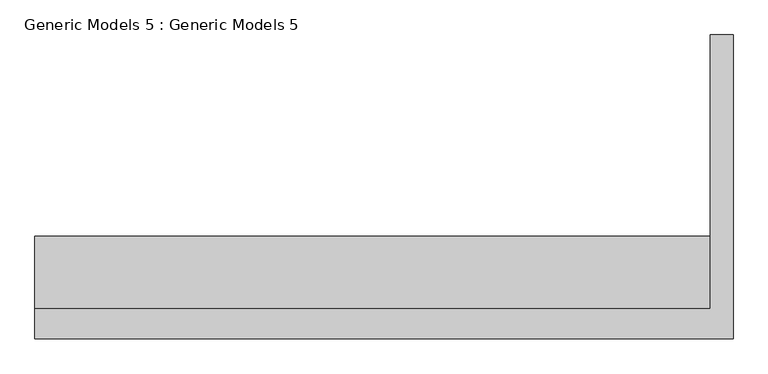
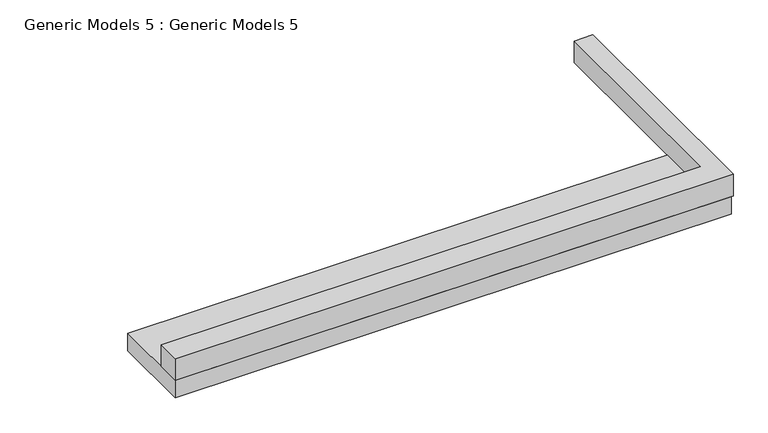
"""IFC4 building model written with IfcOpenShell, lengths in millimetres: proxy geometry, Generic Models 5 : Generic Models 5."""

from ifc_helpers import new_model, si_unit, frame, origin, place, context, project, spatial, polyline, outline, extrude, source, transform, mapped, element, save


def generic_models_5_generic_models_5_36a2ceba(model_context):
    return source(origin(), model_context, "Body", "SweptSolid", [
        extrude(outline(polyline([(-16217.2212454, -15602.9132162), (-16217.2212454, -15171.132201), (-6568.540816, -15171.132201), (-6568.540816, -11258.2252569), (-6239.10287, -11258.2252569), (-6239.10287, -15602.9132162), (-16217.2212454, -15602.9132162)])), frame((0.0, 0.0, 6429.1436541), z_axis=(0.0, 0.0, 1.0), x_axis=(1.0, 0.0, 0.0)), (0.0, 0.0, 1.0), 412.776777),
        extrude(outline(polyline([(-6272.2195233, -15602.9132162), (-16217.2212454, -15602.9132162), (-16217.2212454, -14134.7752569), (-6272.2195233, -14134.7752569), (-6272.2195233, -15602.9132162)])), frame((0.0, 0.0, 6096.0), z_axis=(0.0, 0.0, 1.0), x_axis=(1.0, 0.0, 0.0)), (0.0, 0.0, 1.0), 333.1436541),
    ])


if __name__ == "__main__":
    model = new_model("IFC4")
    model_context = context("Model", 3, world=origin())
    ifc_project = project(units=[si_unit("LENGTHUNIT", "METRE", prefix="MILLI")], contexts=[model_context])
    site = spatial("IfcSite", under=ifc_project)
    building = spatial("IfcBuilding", under=site)
    placement = place(None, origin())
    generic_models_5_generic_models_5_shape = generic_models_5_generic_models_5_36a2ceba(model_context)
    element("IfcBuildingElementProxy", 1, Name="Generic Models 5 : Generic Models 5", ObjectType="Generic Models 5 : Generic Models 5", at=placement, inside=building, context=model_context, shape_type="MappedRepresentation", body=[
        mapped(generic_models_5_generic_models_5_shape, transform((0.0, 0.0, 0.0), x_axis=(1.0, 0.0, 0.0), y_axis=(0.0, 1.0, 0.0), z_axis=(0.0, 0.0, 1.0))),
    ])
    save(model, "model.ifc")
